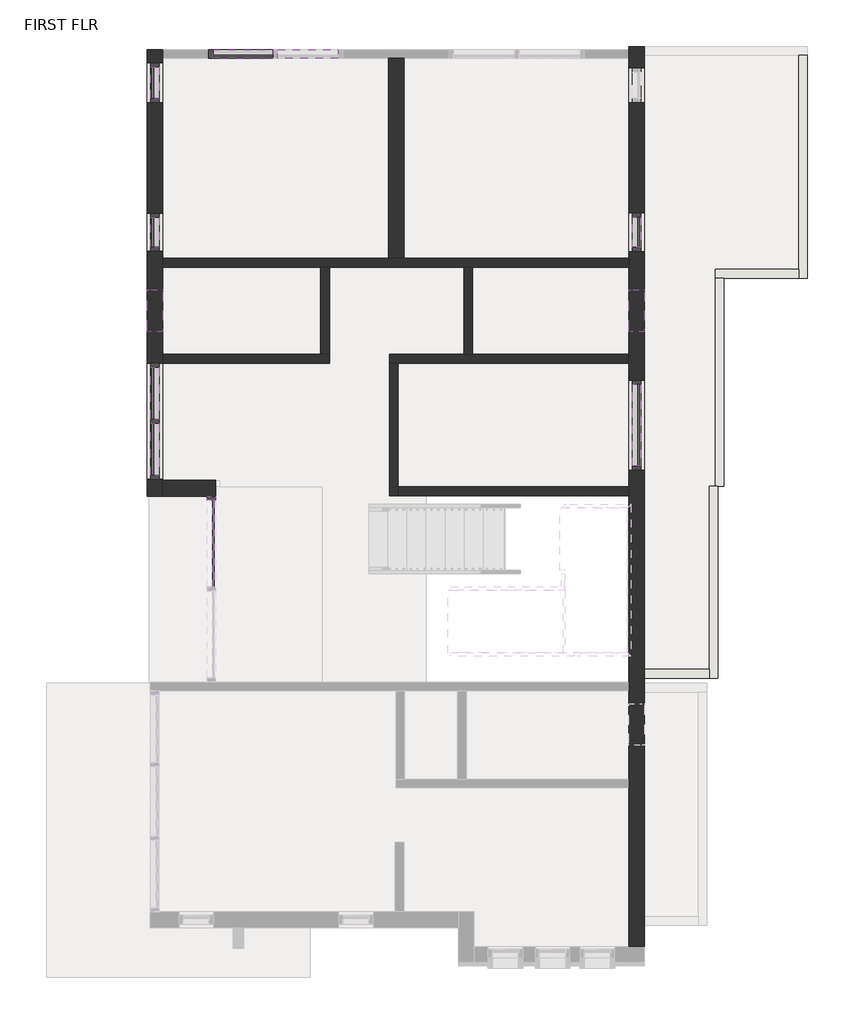
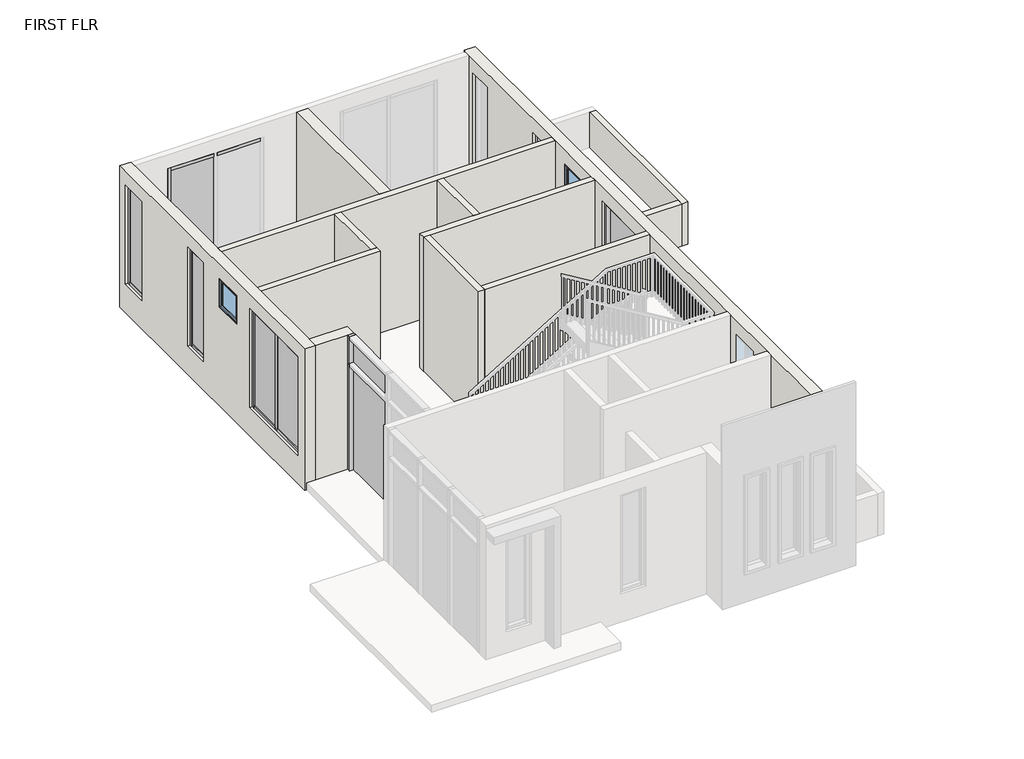
# One storey, part 2 of 4: 30 members, 16 walls, 9 plates, 2 windows.
"""IFC4 building model written with IfcOpenShell, lengths in millimetres."""

from ifc_helpers import new_model, si_unit, frame, origin, place, context, project, spatial, polyline, outline, extrude, faceted_brep, transform, mapped, element, save
from components import member_ee409385, member_2af3cda3, member_47bfaf8a, member_15823cb3, member_69a911c1, member_a3a7b6e3, member_bc7dbe04, member_83167d3d, member_3374d9b6, member_7cbddb58, member_5cd4c5ac, system_panel_glazed_2be43394, system_panel_glazed_82b35773, system_panel_glazed_a1cd5516, system_panel_glazed_0a3516e8, system_panel_glazed_a3b3c321, system_panel_glazed_660eca69, system_panel_glazed_3ab3cb8c, system_panel_glazed_6a2d4635, window_80340324

model = new_model("IFC4")

# Units and contexts
model_context = context("Model", 3, world=origin())
ifc_project = project(units=[si_unit("LENGTHUNIT", "METRE", prefix="MILLI")], contexts=[model_context])

# Site, building, storey
site = spatial("IfcSite", under=ifc_project)
building = spatial("IfcBuilding", under=site)
storey = spatial("IfcBuildingStorey", under=building, Name="FIRST FLR", Elevation=3048.0)

# Members
placement = place(None, origin())
member_shape = member_ee409385(model_context)
element("IfcMember", 1, ObjectType="Rectangular Mullion : 2.5\" x 5\" rectangular", at=placement, inside=storey, context=model_context, shape_type="MappedRepresentation", body=[
    mapped(member_shape, transform((-12015.640556, -5260.3016611, 5486.4), x_axis=(0.0, 1.0, 0.0), y_axis=(-1.0, 0.0, 0.0), z_axis=(0.0, 0.0, 1.0))),
])
member_2_shape = member_2af3cda3(model_context)
element("IfcMember", 2, ObjectType="Rectangular Mullion : 2.5\" x 5\" rectangular", at=placement, inside=storey, context=model_context, shape_type="MappedRepresentation", body=[
    mapped(member_2_shape, transform((-12015.640556, -5323.8016611, 3048.0), x_axis=(0.0, 0.0, -1.0), y_axis=(-1.0, 0.0, 0.0), z_axis=(0.0, 1.0, 0.0))),
])
member_3_shape = member_47bfaf8a(model_context)
element("IfcMember", 3, ObjectType="Rectangular Mullion : 2.5\" x 5\" rectangular", at=placement, inside=storey, context=model_context, shape_type="MappedRepresentation", body=[
    mapped(member_3_shape, transform((-12015.640556, -5260.3016611, 6096.0), x_axis=(0.0, 1.0, 0.0), y_axis=(-1.0, 0.0, 0.0), z_axis=(0.0, 0.0, 1.0))),
])
member_4_shape = member_15823cb3(model_context)
element("IfcMember", 4, ObjectType="Rectangular Mullion : 2.5\" x 5\" rectangular", at=placement, inside=storey, context=model_context, shape_type="MappedRepresentation", body=[
    mapped(member_4_shape, transform((-12841.140556, 556.2983389, 5791.2), x_axis=(0.0, 0.0, 1.0), y_axis=(-1.0, 0.0, 0.0), z_axis=(0.0, -1.0, 0.0))),
])
element("IfcMember", 5, ObjectType="Rectangular Mullion : 2.5\" x 5\" rectangular", at=placement, inside=storey, context=model_context, shape_type="MappedRepresentation", body=[
    mapped(member_4_shape, transform((-12841.140556, 1013.4983389, 3657.6), x_axis=(0.0, 0.0, -1.0), y_axis=(-1.0, 0.0, 0.0), z_axis=(0.0, 1.0, 0.0))),
])
member_5_shape = member_69a911c1(model_context)
element("IfcMember", 6, ObjectType="Rectangular Mullion : 2.5\" x 5\" rectangular", at=placement, inside=storey, context=model_context, shape_type="MappedRepresentation", body=[
    mapped(member_5_shape, transform((-12841.140556, -1617.3738817, 5791.2), x_axis=(0.0, 0.0, 1.0), y_axis=(-1.0, 0.0, 0.0), z_axis=(0.0, -1.0, 0.0))),
])
element("IfcMember", 7, ObjectType="Rectangular Mullion : 2.5\" x 5\" rectangular", at=placement, inside=storey, context=model_context, shape_type="MappedRepresentation", body=[
    mapped(member_5_shape, transform((-12841.140556, -1185.5738817, 3657.6), x_axis=(0.0, 0.0, -1.0), y_axis=(-1.0, 0.0, 0.0), z_axis=(0.0, 1.0, 0.0))),
])
member_6_shape = member_a3a7b6e3(model_context)
element("IfcMember", 8, ObjectType="Rectangular Mullion : 2.5\" x 5\" rectangular", at=placement, inside=storey, context=model_context, shape_type="MappedRepresentation", body=[
    mapped(member_6_shape, transform((-12841.140556, -4953.7451712, 5791.2), x_axis=(0.0, 0.0, 1.0), y_axis=(-1.0, 0.0, 0.0), z_axis=(0.0, -1.0, 0.0))),
])
element("IfcMember", 9, ObjectType="Rectangular Mullion : 2.5\" x 5\" rectangular", at=placement, inside=storey, context=model_context, shape_type="MappedRepresentation", body=[
    mapped(member_6_shape, transform((-12841.140556, -4134.5951712, 5791.2), x_axis=(0.0, 0.0, 1.0), y_axis=(-1.0, 0.0, 0.0), z_axis=(0.0, -1.0, 0.0))),
])
element("IfcMember", 10, ObjectType="Rectangular Mullion : 2.5\" x 5\" rectangular", at=placement, inside=storey, context=model_context, shape_type="MappedRepresentation", body=[
    mapped(member_6_shape, transform((-12841.140556, -3378.9451712, 3657.6), x_axis=(0.0, 0.0, -1.0), y_axis=(-1.0, 0.0, 0.0), z_axis=(0.0, 1.0, 0.0))),
])
element("IfcMember", 11, ObjectType="Rectangular Mullion : 2.5\" x 5\" rectangular", at=placement, inside=storey, context=model_context, shape_type="MappedRepresentation", body=[
    mapped(member_6_shape, transform((-12841.140556, -4198.0951712, 3657.6), x_axis=(0.0, 0.0, -1.0), y_axis=(-1.0, 0.0, 0.0), z_axis=(0.0, 1.0, 0.0))),
])
member_7_shape = member_bc7dbe04(model_context)
element("IfcMember", 12, ObjectType="Rectangular Mullion : 2.5\" x 5\" rectangular", at=placement, inside=storey, context=model_context, shape_type="MappedRepresentation", body=[
    mapped(member_7_shape, transform((-5795.8906521, -1625.1830995, 5791.2), x_axis=(0.0, 0.0, 1.0), y_axis=(-1.0, 0.0, 0.0), z_axis=(0.0, -1.0, 0.0))),
])
element("IfcMember", 13, ObjectType="Rectangular Mullion : 2.5\" x 5\" rectangular", at=placement, inside=storey, context=model_context, shape_type="MappedRepresentation", body=[
    mapped(member_7_shape, transform((-5795.8906521, -1180.6830995, 3657.6), x_axis=(0.0, 0.0, -1.0), y_axis=(-1.0, 0.0, 0.0), z_axis=(0.0, 1.0, 0.0))),
])
member_8_shape = member_83167d3d(model_context)
element("IfcMember", 14, ObjectType="Rectangular Mullion : 2.5\" x 5\" rectangular", at=placement, inside=storey, context=model_context, shape_type="MappedRepresentation", body=[
    mapped(member_8_shape, transform((-5795.8906521, -3626.5951712, 5791.2), x_axis=(0.0, 0.0, 1.0), y_axis=(1.0, 0.0, 0.0), z_axis=(0.0, 1.0, 0.0))),
])
element("IfcMember", 15, ObjectType="Rectangular Mullion : 2.5\" x 5\" rectangular", at=placement, inside=storey, context=model_context, shape_type="MappedRepresentation", body=[
    mapped(member_8_shape, transform((-5795.8906521, -4820.3951712, 3657.6), x_axis=(0.0, 0.0, -1.0), y_axis=(1.0, 0.0, 0.0), z_axis=(0.0, -1.0, 0.0))),
])
member_9_shape = member_3374d9b6(model_context)
element("IfcMember", 16, ObjectType="Rectangular Mullion : 2.5\" x 5\" rectangular", at=placement, inside=storey, context=model_context, shape_type="MappedRepresentation", body=[
    mapped(member_9_shape, transform((-12841.140556, 492.7983389, 3657.6), x_axis=(0.0, -1.0, 0.0), y_axis=(-1.0, 0.0, 0.0), z_axis=(0.0, 0.0, -1.0))),
])
element("IfcMember", 17, ObjectType="Rectangular Mullion : 2.5\" x 5\" rectangular", at=placement, inside=storey, context=model_context, shape_type="MappedRepresentation", body=[
    mapped(member_9_shape, transform((-12841.140556, -1680.8738817, 3657.6), x_axis=(0.0, -1.0, 0.0), y_axis=(-1.0, 0.0, 0.0), z_axis=(0.0, 0.0, -1.0))),
])
element("IfcMember", 18, ObjectType="Rectangular Mullion : 2.5\" x 5\" rectangular", at=placement, inside=storey, context=model_context, shape_type="MappedRepresentation", body=[
    mapped(member_9_shape, transform((-12841.140556, -5017.2451712, 3657.6), x_axis=(0.0, -1.0, 0.0), y_axis=(-1.0, 0.0, 0.0), z_axis=(0.0, 0.0, -1.0))),
])
element("IfcMember", 19, ObjectType="Rectangular Mullion : 2.5\" x 5\" rectangular", at=placement, inside=storey, context=model_context, shape_type="MappedRepresentation", body=[
    mapped(member_9_shape, transform((-5795.8906521, -3563.0951712, 3657.6), x_axis=(0.0, 1.0, 0.0), y_axis=(1.0, 0.0, 0.0), z_axis=(0.0, 0.0, -1.0))),
])
element("IfcMember", 20, ObjectType="Rectangular Mullion : 2.5\" x 5\" rectangular", at=placement, inside=storey, context=model_context, shape_type="MappedRepresentation", body=[
    mapped(member_9_shape, transform((-12841.140556, 1076.9983389, 5791.2), x_axis=(0.0, 1.0, 0.0), y_axis=(-1.0, 0.0, 0.0), z_axis=(0.0, 0.0, 1.0))),
])
element("IfcMember", 21, ObjectType="Rectangular Mullion : 2.5\" x 5\" rectangular", at=placement, inside=storey, context=model_context, shape_type="MappedRepresentation", body=[
    mapped(member_9_shape, transform((-12841.140556, -1122.0738817, 5791.2), x_axis=(0.0, 1.0, 0.0), y_axis=(-1.0, 0.0, 0.0), z_axis=(0.0, 0.0, 1.0))),
])
element("IfcMember", 22, ObjectType="Rectangular Mullion : 2.5\" x 5\" rectangular", at=placement, inside=storey, context=model_context, shape_type="MappedRepresentation", body=[
    mapped(member_9_shape, transform((-12841.140556, -3315.4451712, 5791.2), x_axis=(0.0, 1.0, 0.0), y_axis=(-1.0, 0.0, 0.0), z_axis=(0.0, 0.0, 1.0))),
])
element("IfcMember", 23, ObjectType="Rectangular Mullion : 2.5\" x 5\" rectangular", at=placement, inside=storey, context=model_context, shape_type="MappedRepresentation", body=[
    mapped(member_9_shape, transform((-5795.8906521, -4883.8951712, 5791.2), x_axis=(0.0, -1.0, 0.0), y_axis=(1.0, 0.0, 0.0), z_axis=(0.0, 0.0, 1.0))),
])
member_10_shape = member_7cbddb58(model_context)
element("IfcMember", 24, ObjectType="Rectangular Mullion : 2.5\" x 5\" rectangular", at=placement, inside=storey, context=model_context, shape_type="MappedRepresentation", body=[
    mapped(member_10_shape, transform((-12841.140556, -4166.3451712, 3657.6), x_axis=(0.0, -1.0, 0.0), y_axis=(-1.0, 0.0, 0.0), z_axis=(0.0, 0.0, -1.0))),
])
element("IfcMember", 25, ObjectType="Rectangular Mullion : 2.5\" x 5\" rectangular", at=placement, inside=storey, context=model_context, shape_type="MappedRepresentation", body=[
    mapped(member_9_shape, transform((-5795.8906521, -1688.6830995, 3657.6), x_axis=(0.0, -1.0, 0.0), y_axis=(-1.0, 0.0, 0.0), z_axis=(0.0, 0.0, -1.0))),
])
element("IfcMember", 26, ObjectType="Rectangular Mullion : 2.5\" x 5\" rectangular", at=placement, inside=storey, context=model_context, shape_type="MappedRepresentation", body=[
    mapped(member_9_shape, transform((-12054.1911408, 1203.9983389, 3657.6), x_axis=(-1.0, 0.0, 0.0), y_axis=(0.0, 1.0, 0.0), z_axis=(0.0, 0.0, -1.0))),
])
element("IfcMember", 27, ObjectType="Rectangular Mullion : 2.5\" x 5\" rectangular", at=placement, inside=storey, context=model_context, shape_type="MappedRepresentation", body=[
    mapped(member_9_shape, transform((-5795.8906521, -1117.1830995, 5791.2), x_axis=(0.0, 1.0, 0.0), y_axis=(-1.0, 0.0, 0.0), z_axis=(0.0, 0.0, 1.0))),
])
member_11_shape = member_5cd4c5ac(model_context)
element("IfcMember", 28, ObjectType="Rectangular Mullion : 2.5\" x 5\" rectangular", at=placement, inside=storey, context=model_context, shape_type="MappedRepresentation", body=[
    mapped(member_11_shape, transform((-11990.6911408, 1203.9983389, 5791.2), x_axis=(0.0, 0.0, 1.0), y_axis=(0.0, 1.0, 0.0), z_axis=(-1.0, 0.0, 0.0))),
])
element("IfcMember", 29, ObjectType="Rectangular Mullion : 2.5\" x 5\" rectangular", at=placement, inside=storey, context=model_context, shape_type="MappedRepresentation", body=[
    mapped(member_11_shape, transform((-11044.5411408, 1203.9983389, 5791.2), x_axis=(0.0, 0.0, 1.0), y_axis=(0.0, 1.0, 0.0), z_axis=(-1.0, 0.0, 0.0))),
])
element("IfcMember", 30, ObjectType="Rectangular Mullion : 2.5\" x 5\" rectangular", at=placement, inside=storey, context=model_context, shape_type="MappedRepresentation", body=[
    mapped(member_11_shape, transform((-11108.0411408, 1203.9983389, 3657.6), x_axis=(0.0, 0.0, -1.0), y_axis=(0.0, 1.0, 0.0), z_axis=(1.0, 0.0, 0.0))),
])

# Plates
system_panel_glazed_shape = system_panel_glazed_2be43394(model_context)
element("IfcPlate", 31, ObjectType="System Panel : Glazed", at=placement, inside=storey, context=model_context, shape_type="MappedRepresentation", body=[
    mapped(system_panel_glazed_shape, transform((-12015.640556, -5955.8340156, 3111.5), x_axis=(0.0, -1.0, 0.0), y_axis=(1.0, 0.0, 0.0), z_axis=(0.0, 0.0, 1.0))),
])
system_panel_glazed_2_shape = system_panel_glazed_82b35773(model_context)
element("IfcPlate", 32, ObjectType="System Panel : Glazed", at=placement, inside=storey, context=model_context, shape_type="MappedRepresentation", body=[
    mapped(system_panel_glazed_2_shape, transform((-12015.640556, -5955.8340156, 5518.15), x_axis=(0.0, -1.0, 0.0), y_axis=(1.0, 0.0, 0.0), z_axis=(0.0, 0.0, 1.0))),
])
system_panel_glazed_3_shape = system_panel_glazed_a1cd5516(model_context)
element("IfcPlate", 33, ObjectType="System Panel : Glazed", at=placement, inside=storey, context=model_context, shape_type="MappedRepresentation", body=[
    mapped(system_panel_glazed_3_shape, transform((-12841.140556, 784.8983389, 3721.1), x_axis=(0.0, -1.0, 0.0), y_axis=(1.0, 0.0, 0.0), z_axis=(0.0, 0.0, 1.0))),
])
system_panel_glazed_4_shape = system_panel_glazed_0a3516e8(model_context)
element("IfcPlate", 34, ObjectType="System Panel : Glazed", at=placement, inside=storey, context=model_context, shape_type="MappedRepresentation", body=[
    mapped(system_panel_glazed_4_shape, transform((-12841.140556, -1401.4738817, 3721.1), x_axis=(0.0, -1.0, 0.0), y_axis=(1.0, 0.0, 0.0), z_axis=(0.0, 0.0, 1.0))),
])
system_panel_glazed_5_shape = system_panel_glazed_a3b3c321(model_context)
element("IfcPlate", 35, ObjectType="System Panel : Glazed", at=placement, inside=storey, context=model_context, shape_type="MappedRepresentation", body=[
    mapped(system_panel_glazed_5_shape, transform((-12841.140556, -3756.7701712, 3721.1), x_axis=(0.0, -1.0, 0.0), y_axis=(1.0, 0.0, 0.0), z_axis=(0.0, 0.0, 1.0))),
])
element("IfcPlate", 36, ObjectType="System Panel : Glazed", at=placement, inside=storey, context=model_context, shape_type="MappedRepresentation", body=[
    mapped(system_panel_glazed_5_shape, transform((-12841.140556, -4575.9201712, 3721.1), x_axis=(0.0, -1.0, 0.0), y_axis=(1.0, 0.0, 0.0), z_axis=(0.0, 0.0, 1.0))),
])
system_panel_glazed_6_shape = system_panel_glazed_660eca69(model_context)
element("IfcPlate", 37, ObjectType="System Panel : Glazed", at=placement, inside=storey, context=model_context, shape_type="MappedRepresentation", body=[
    mapped(system_panel_glazed_6_shape, transform((-5795.8906521, -1402.9330995, 3721.1), x_axis=(0.0, -1.0, 0.0), y_axis=(1.0, 0.0, 0.0), z_axis=(0.0, 0.0, 1.0))),
])
system_panel_glazed_7_shape = system_panel_glazed_3ab3cb8c(model_context)
element("IfcPlate", 38, ObjectType="System Panel : Glazed", at=placement, inside=storey, context=model_context, shape_type="MappedRepresentation", body=[
    mapped(system_panel_glazed_7_shape, transform((-11549.3661408, 1203.9983389, 3721.1), x_axis=(-1.0, 0.0, 0.0), y_axis=(0.0, -1.0, 0.0), z_axis=(0.0, 0.0, 1.0))),
])
system_panel_glazed_8_shape = system_panel_glazed_6a2d4635(model_context)
element("IfcPlate", 39, ObjectType="System Panel : Glazed", at=placement, inside=storey, context=model_context, shape_type="MappedRepresentation", body=[
    mapped(system_panel_glazed_8_shape, transform((-5795.8906521, -4223.4951712, 3721.1), x_axis=(0.0, 1.0, 0.0), y_axis=(-1.0, 0.0, 0.0), z_axis=(0.0, 0.0, 1.0))),
])

# Walls
element("IfcWall", 40, ObjectType="EXTERIOR WALL 9\"", at=placement, inside=storey, context=model_context, shape_type="Brep", body=[
    faceted_brep([(-12955.440556, 1267.4983389, 3048.0), (-12955.440556, -5260.3016611, 3048.0), (-12955.440556, -5260.3016611, 6096.0), (-12955.440556, 1267.4983389, 6096.0), (-12955.440556, 1076.9983389, 3657.6), (-12955.440556, 1076.9983389, 5791.2), (-12955.440556, 492.7983389, 5791.2), (-12955.440556, 492.7983389, 3657.6), (-12955.440556, -1122.0738817, 3657.6), (-12955.440556, -1122.0738817, 5791.2), (-12955.440556, -1680.8738817, 5791.2), (-12955.440556, -1680.8738817, 3657.6), (-12955.440556, -3315.4451712, 3657.6), (-12955.440556, -3315.4451712, 5791.2), (-12955.440556, -5017.2451712, 5791.2), (-12955.440556, -5017.2451712, 3657.6), (-12955.440556, -2245.4701712, 5791.2), (-12955.440556, -2855.0701712, 5791.2), (-12955.440556, -2855.0701712, 5181.6), (-12955.440556, -2245.4701712, 5181.6), (-12726.840556, -5260.3016611, 3048.0), (-12726.840556, -5031.7016611, 3048.0), (-12726.840556, -3315.4451712, 3048.0), (-12726.840556, -3188.4451712, 3048.0), (-12726.840556, -1912.0951712, 3048.0), (-12726.840556, -1785.0951712, 3048.0), (-12726.840556, 1140.4983389, 3048.0), (-12726.840556, 1267.4983389, 3048.0), (-12726.840556, 1267.4983389, 6096.0), (-12726.840556, 1140.4983389, 6096.0), (-12726.840556, -1785.0951712, 6096.0), (-12726.840556, -1912.0951712, 6096.0), (-12726.840556, -3188.4451712, 6096.0), (-12726.840556, -3315.4451712, 6096.0), (-12726.840556, -5031.7016611, 6096.0), (-12726.840556, -5260.3016611, 6096.0), (-12726.840556, 1076.9983389, 5791.2), (-12726.840556, 1076.9983389, 3657.6), (-12726.840556, 492.7983389, 3657.6), (-12726.840556, 492.7983389, 5791.2), (-12726.840556, -1122.0738817, 5791.2), (-12726.840556, -1122.0738817, 3657.6), (-12726.840556, -1680.8738817, 3657.6), (-12726.840556, -1680.8738817, 5791.2), (-12726.840556, -3315.4451712, 5791.2), (-12726.840556, -3315.4451712, 3657.6), (-12726.840556, -5017.2451712, 3657.6), (-12726.840556, -5017.2451712, 5791.2), (-12726.840556, -2245.4701712, 5791.2), (-12726.840556, -2245.4701712, 5181.6), (-12726.840556, -2855.0701712, 5181.6), (-12726.840556, -2855.0701712, 5791.2)], [[[0, 1, 2, 3], [4, 5, 6, 7], [8, 9, 10, 11], [12, 13, 14, 15], [16, 17, 18, 19]], [[20, 21, 22, 23, 24, 25, 26, 27, 28, 29, 30, 31, 32, 33, 34, 35], [36, 37, 38, 39], [40, 41, 42, 43], [44, 45, 46, 47], [48, 49, 50, 51]], [[1, 0, 27, 26, 25, 24, 23, 22, 21, 20]], [[3, 2, 35, 34, 33, 32, 31, 30, 29, 28]], [[2, 1, 20, 35]], [[0, 3, 28, 27]], [[36, 5, 4, 37]], [[5, 36, 39, 6]], [[6, 39, 38, 7]], [[37, 4, 7, 38]], [[8, 41, 40, 9]], [[9, 40, 43, 10]], [[10, 43, 42, 11]], [[41, 8, 11, 42]], [[12, 45, 44, 13]], [[13, 44, 47, 14]], [[46, 15, 14, 47]], [[45, 12, 15, 46]], [[49, 48, 16, 19]], [[50, 49, 19, 18]], [[51, 50, 18, 17]], [[48, 51, 17, 16]]]),
])
element("IfcWall", 41, ObjectType="EXTERIOR WALL 9\"", at=placement, inside=storey, context=model_context, shape_type="SweptSolid", body=[
    extrude(outline(polyline([(-11952.140556, -5260.3016611), (-12726.840556, -5260.3016611), (-12726.840556, -5031.7016611), (-11952.140556, -5031.7016611), (-11952.140556, -5260.3016611)])), frame((0.0, 0.0, 3048.0), z_axis=(0.0, 0.0, 1.0), x_axis=(1.0, 0.0, 0.0)), (0.0, 0.0, 1.0), 3048.0),
])
element("IfcWall", 42, ObjectType="EXTERIOR WALL 9\"", at=placement, inside=storey, context=model_context, shape_type="Brep", body=[
    faceted_brep([(-5681.5906521, -11847.6453012, 3048.0), (-5681.5906521, -11534.9310793, 3048.0), (-5681.5906521, -11407.9310793, 3048.0), (-5681.5906521, -8124.9810793, 3048.0), (-5681.5906521, -7997.9810793, 3048.0), (-5681.5906521, -7921.7810793, 3048.0), (-5681.5906521, -7794.7810793, 3048.0), (-5681.5906521, 1184.7951326, 3048.0), (-5681.5906521, 1311.7951326, 3048.0), (-5681.5906521, 1311.7951326, 3962.4), (-5681.5906521, 1311.7951326, 6096.0), (-5681.5906521, -11847.6453012, 6096.0), (-5681.5906521, 1000.7983389, 5791.2), (-5681.5906521, 1000.7983389, 3657.6), (-5681.5906521, 492.7983389, 3657.6), (-5681.5906521, 492.7983389, 5791.2), (-5681.5906521, -1117.1830995, 5791.2), (-5681.5906521, -1117.1830995, 3657.6), (-5681.5906521, -1688.6830995, 3657.6), (-5681.5906521, -1688.6830995, 5791.2), (-5681.5906521, -2245.4701712, 5791.2), (-5681.5906521, -2245.4701712, 5181.6), (-5681.5906521, -2855.0701712, 5181.6), (-5681.5906521, -2855.0701712, 5791.2), (-5681.5906521, -4883.8951712, 3657.6), (-5681.5906521, -4883.8951712, 5791.2), (-5681.5906521, -3563.0951712, 5791.2), (-5681.5906521, -3563.0951712, 3657.6), (-5681.5906521, -8906.0310793, 5791.2), (-5681.5906521, -8296.4310793, 5791.2), (-5681.5906521, -8296.4310793, 5181.6), (-5681.5906521, -8906.0310793, 5181.6), (-5910.1906521, 1311.7951326, 3048.0), (-5910.1906521, 1267.4983389, 3048.0), (-5910.1906521, 1140.4983389, 3048.0), (-5910.1906521, -1785.0951712, 3048.0), (-5910.1906521, -1912.0951712, 3048.0), (-5910.1906521, -3188.4451712, 3048.0), (-5910.1906521, -3315.4451712, 3048.0), (-5910.1906521, -5125.1951712, 3048.0), (-5910.1906521, -5252.1951712, 3048.0), (-5910.1906521, -7978.9310793, 3048.0), (-5910.1906521, -8105.9310793, 3048.0), (-5910.1906521, -9397.5830995, 3048.0), (-5910.1906521, -9524.5830995, 3048.0), (-5910.1906521, -11847.6453012, 3048.0), (-5910.1906521, -11847.6453012, 6096.0), (-5910.1906521, -9524.5830995, 6096.0), (-5910.1906521, -9397.5830995, 6096.0), (-5910.1906521, -8105.9310793, 6096.0), (-5910.1906521, -7978.9310793, 6096.0), (-5910.1906521, -5252.1951712, 6096.0), (-5910.1906521, -5125.1951712, 6096.0), (-5910.1906521, -3315.4451712, 6096.0), (-5910.1906521, -3188.4451712, 6096.0), (-5910.1906521, -1912.0951712, 6096.0), (-5910.1906521, -1785.0951712, 6096.0), (-5910.1906521, 1140.4983389, 6096.0), (-5910.1906521, 1267.4983389, 6096.0), (-5910.1906521, 1311.7951326, 6096.0), (-5910.1906521, 1000.7983389, 3657.6), (-5910.1906521, 1000.7983389, 5791.2), (-5910.1906521, 492.7983389, 5791.2), (-5910.1906521, 492.7983389, 3657.6), (-5910.1906521, -1117.1830995, 3657.6), (-5910.1906521, -1117.1830995, 5791.2), (-5910.1906521, -1688.6830995, 5791.2), (-5910.1906521, -1688.6830995, 3657.6), (-5910.1906521, -2245.4701712, 5791.2), (-5910.1906521, -2855.0701712, 5791.2), (-5910.1906521, -2855.0701712, 5181.6), (-5910.1906521, -2245.4701712, 5181.6), (-5910.1906521, -4883.8951712, 5791.2), (-5910.1906521, -4883.8951712, 3657.6), (-5910.1906521, -3563.0951712, 3657.6), (-5910.1906521, -3563.0951712, 5791.2), (-5910.1906521, -8906.0310793, 5791.2), (-5910.1906521, -8906.0310793, 5181.6), (-5910.1906521, -8296.4310793, 5181.6), (-5910.1906521, -8296.4310793, 5791.2)], [[[0, 1, 2, 3, 4, 5, 6, 7, 8, 9, 10, 11], [12, 13, 14, 15], [16, 17, 18, 19], [20, 21, 22, 23], [24, 25, 26, 27], [28, 29, 30, 31]], [[32, 33, 34, 35, 36, 37, 38, 39, 40, 41, 42, 43, 44, 45, 46, 47, 48, 49, 50, 51, 52, 53, 54, 55, 56, 57, 58, 59], [60, 61, 62, 63], [64, 65, 66, 67], [68, 69, 70, 71], [72, 73, 74, 75], [76, 77, 78, 79]], [[8, 7, 6, 5, 4, 3, 2, 1, 0, 45, 44, 43, 42, 41, 40, 39, 38, 37, 36, 35, 34, 33, 32]], [[11, 10, 59, 58, 57, 56, 55, 54, 53, 52, 51, 50, 49, 48, 47, 46]], [[0, 11, 46, 45]], [[12, 61, 60, 13]], [[61, 12, 15, 62]], [[62, 15, 14, 63]], [[13, 60, 63, 14]], [[64, 17, 16, 65]], [[65, 16, 19, 66]], [[66, 19, 18, 67]], [[17, 64, 67, 18]], [[21, 20, 68, 71]], [[22, 21, 71, 70]], [[23, 22, 70, 69]], [[20, 23, 69, 68]], [[72, 25, 24, 73]], [[25, 72, 75, 26]], [[26, 75, 74, 27]], [[73, 24, 27, 74]], [[77, 76, 28, 31]], [[78, 77, 31, 30]], [[79, 78, 30, 29]], [[76, 79, 29, 28]], [[10, 9, 8, 32, 59]]]),
])
element("IfcWall", 43, ObjectType="EXTERIOR WALL 9\"", at=placement, inside=storey, context=model_context, shape_type="SweptSolid", body=[
    extrude(outline(polyline([(-9425.2911408, -1785.0951712), (-9425.2911408, 1140.4983389), (-9196.6911408, 1140.4983389), (-9196.6911408, -1785.0951712), (-9425.2911408, -1785.0951712)])), frame((0.0, 0.0, 3048.0), z_axis=(0.0, 0.0, 1.0), x_axis=(1.0, 0.0, 0.0)), (0.0, 0.0, 1.0), 3048.0),
])
element("IfcWall", 44, ObjectType="INTERIOR WALL PAINT 5\"", at=placement, inside=storey, context=model_context, shape_type="Brep", body=[
    faceted_brep([(-12726.840556, -1912.0951712, 3048.0), (-10415.440556, -1912.0951712, 3048.0), (-10288.440556, -1912.0951712, 3048.0), (-8320.3911408, -1912.0951712, 3048.0), (-8193.3911408, -1912.0951712, 3048.0), (-5910.1906521, -1912.0951712, 3048.0), (-5910.1906521, -1912.0951712, 6096.0), (-8193.3911408, -1912.0951712, 6096.0), (-8320.3911408, -1912.0951712, 6096.0), (-10288.440556, -1912.0951712, 6096.0), (-10415.440556, -1912.0951712, 6096.0), (-12726.840556, -1912.0951712, 6096.0), (-12726.840556, -1785.0951712, 3048.0), (-12726.840556, -1785.0951712, 6096.0), (-9425.2911408, -1785.0951712, 6096.0), (-9196.6911408, -1785.0951712, 6096.0), (-5910.1906521, -1785.0951712, 6096.0), (-5910.1906521, -1785.0951712, 3048.0), (-9196.6911408, -1785.0951712, 3048.0), (-9425.2911408, -1785.0951712, 3048.0)], [[[0, 1, 2, 3, 4, 5, 6, 7, 8, 9, 10, 11]], [[12, 13, 14, 15, 16, 17, 18, 19]], [[5, 4, 3, 2, 1, 0, 12, 19, 18, 17]], [[11, 10, 9, 8, 7, 6, 16, 15, 14, 13]], [[0, 11, 13, 12]], [[6, 5, 17, 16]]]),
])
element("IfcWall", 45, ObjectType="INTERIOR WALL PAINT 5\"", at=placement, inside=storey, context=model_context, shape_type="Brep", body=[
    faceted_brep([(-12726.840556, -3315.4451712, 3048.0), (-10288.440556, -3315.4451712, 3048.0), (-10288.440556, -3315.4451712, 6096.0), (-12726.840556, -3315.4451712, 6096.0), (-12726.840556, -3188.4451712, 3048.0), (-12726.840556, -3188.4451712, 6096.0), (-10415.440556, -3188.4451712, 6096.0), (-10288.440556, -3188.4451712, 6096.0), (-10288.440556, -3188.4451712, 3048.0), (-10415.440556, -3188.4451712, 3048.0)], [[[0, 1, 2, 3]], [[4, 5, 6, 7, 8, 9]], [[1, 0, 4, 9, 8]], [[3, 2, 7, 6, 5]], [[0, 3, 5, 4]], [[2, 1, 8, 7]]]),
])
element("IfcWall", 46, ObjectType="INTERIOR WALL PAINT 5\"", at=placement, inside=storey, context=model_context, shape_type="SweptSolid", body=[
    extrude(outline(polyline([(-10288.440556, -1912.0951712), (-10288.440556, -3188.4451712), (-10415.440556, -3188.4451712), (-10415.440556, -1912.0951712), (-10288.440556, -1912.0951712)])), frame((0.0, 0.0, 3048.0), z_axis=(0.0, 0.0, 1.0), x_axis=(1.0, 0.0, 0.0)), (0.0, 0.0, 1.0), 3048.0),
])
element("IfcWall", 47, ObjectType="INTERIOR WALL PAINT 5\"", at=placement, inside=storey, context=model_context, shape_type="Brep", body=[
    faceted_brep([(-5910.1906521, -3188.4451712, 3048.0), (-8193.3911408, -3188.4451712, 3048.0), (-8320.3911408, -3188.4451712, 3048.0), (-9409.0406521, -3188.4451712, 3048.0), (-9409.0406521, -3188.4451712, 6096.0), (-8320.3911408, -3188.4451712, 6096.0), (-8193.3911408, -3188.4451712, 6096.0), (-5910.1906521, -3188.4451712, 6096.0), (-5910.1906521, -3315.4451712, 3048.0), (-5910.1906521, -3315.4451712, 6096.0), (-9282.0406521, -3315.4451712, 6096.0), (-9409.0406521, -3315.4451712, 6096.0), (-9409.0406521, -3315.4451712, 3048.0), (-9282.0406521, -3315.4451712, 3048.0)], [[[0, 1, 2, 3, 4, 5, 6, 7]], [[8, 9, 10, 11, 12, 13]], [[3, 2, 1, 0, 8, 13, 12]], [[7, 6, 5, 4, 11, 10, 9]], [[0, 7, 9, 8]], [[4, 3, 12, 11]]]),
])
element("IfcWall", 48, ObjectType="INTERIOR WALL PAINT 5\"", at=placement, inside=storey, context=model_context, shape_type="SweptSolid", body=[
    extrude(outline(polyline([(-8320.3911408, -3188.4451712), (-8320.3911408, -1912.0951712), (-8193.3911408, -1912.0951712), (-8193.3911408, -3188.4451712), (-8320.3911408, -3188.4451712)])), frame((0.0, 0.0, 3048.0), z_axis=(0.0, 0.0, 1.0), x_axis=(1.0, 0.0, 0.0)), (0.0, 0.0, 1.0), 3048.0),
])
element("IfcWall", 49, ObjectType="INTERIOR WALL PAINT 5\"", at=placement, inside=storey, context=model_context, shape_type="Brep", body=[
    faceted_brep([(-9409.0406521, -3315.4451712, 3048.0), (-9409.0406521, -5252.1951712, 3048.0), (-9409.0406521, -5252.1951712, 6096.0), (-9409.0406521, -3315.4451712, 6096.0), (-9282.0406521, -3315.4451712, 3048.0), (-9282.0406521, -3315.4451712, 6096.0), (-9282.0406521, -5125.1951712, 6096.0), (-9282.0406521, -5252.1951712, 6096.0), (-9282.0406521, -5252.1951712, 3048.0), (-9282.0406521, -5125.1951712, 3048.0)], [[[0, 1, 2, 3]], [[4, 5, 6, 7, 8, 9]], [[1, 0, 4, 9, 8]], [[3, 2, 7, 6, 5]], [[0, 3, 5, 4]], [[2, 1, 8, 7]]]),
])
element("IfcWall", 50, ObjectType="INTERIOR WALL PAINT 5\"", at=placement, inside=storey, context=model_context, shape_type="SweptSolid", body=[
    extrude(outline(polyline([(-5910.1906521, -5252.1951712), (-9282.0406521, -5252.1951712), (-9282.0406521, -5125.1951712), (-5910.1906521, -5125.1951712), (-5910.1906521, -5252.1951712)])), frame((0.0, 0.0, 3048.0), z_axis=(0.0, 0.0, 1.0), x_axis=(1.0, 0.0, 0.0)), (0.0, 0.0, 1.0), 3048.0),
])
element("IfcWall", 51, ObjectType="INTERIOR WALL PAINT 5\"", at=placement, inside=storey, context=model_context, shape_type="Brep", body=[
    faceted_brep([(-3424.4727979, 1184.7951326, 3048.0), (-3424.4727979, -1944.8337491, 3048.0), (-3424.4727979, -2071.8337491, 3048.0), (-3424.4727979, -2071.8337491, 3962.4), (-3424.4727979, -1944.8337491, 3962.4), (-3424.4727979, 1184.7951326, 3962.4), (-3297.4727979, 1184.7951326, 3048.0), (-3297.4727979, 1184.7951326, 3962.4), (-3297.4727979, -2071.8337491, 3962.4), (-3297.4727979, -2071.8337491, 3048.0)], [[[0, 1, 2, 3, 4, 5]], [[6, 7, 8, 9]], [[2, 1, 0, 6, 9]], [[5, 4, 3, 8, 7]], [[0, 5, 7, 6]], [[3, 2, 9, 8]]]),
])
element("IfcWall", 52, ObjectType="INTERIOR WALL PAINT 5\"", at=placement, inside=storey, context=model_context, shape_type="Brep", body=[
    faceted_brep([(-3424.4727979, -1944.8337491, 3048.0), (-4643.6727979, -1944.8337491, 3048.0), (-4643.6727979, -1944.8337491, 3962.4), (-3424.4727979, -1944.8337491, 3962.4), (-3424.4727979, -2071.8337491, 3048.0), (-3424.4727979, -2071.8337491, 3962.4), (-4516.6727979, -2071.8337491, 3962.4), (-4643.6727979, -2071.8337491, 3962.4), (-4643.6727979, -2071.8337491, 3048.0), (-4516.6727979, -2071.8337491, 3048.0)], [[[0, 1, 2, 3]], [[4, 5, 6, 7, 8, 9]], [[1, 0, 4, 9, 8]], [[3, 2, 7, 6, 5]], [[0, 3, 5, 4]], [[2, 1, 8, 7]]]),
])
element("IfcWall", 53, ObjectType="INTERIOR WALL PAINT 5\"", at=placement, inside=storey, context=model_context, shape_type="Brep", body=[
    faceted_brep([(-4643.6727979, -2071.8337491, 3048.0), (-4643.6727979, -5119.6951024, 3048.0), (-4643.6727979, -5119.6951024, 3962.4), (-4643.6727979, -2071.8337491, 3962.4), (-4516.6727979, -2071.8337491, 3048.0), (-4516.6727979, -2071.8337491, 3962.4), (-4516.6727979, -5119.6951024, 3962.4), (-4516.6727979, -5119.6951024, 3048.0), (-4605.5727979, -5119.6951024, 3048.0), (-4605.5727979, -5119.6951024, 3962.4)], [[[0, 1, 2, 3]], [[4, 5, 6, 7]], [[1, 0, 4, 7, 8]], [[2, 1, 8, 7, 6, 9]], [[3, 2, 9, 6, 5]], [[0, 3, 5, 4]]]),
])
element("IfcWall", 54, ObjectType="INTERIOR WALL PAINT 5\"", at=placement, inside=storey, context=model_context, shape_type="Brep", body=[
    faceted_brep([(-4732.5727979, -5119.6951024, 3048.0), (-4732.5727979, -7794.7810793, 3048.0), (-4732.5727979, -7921.7810793, 3048.0), (-4732.5727979, -7921.7810793, 3962.4), (-4732.5727979, -7794.7810793, 3962.4), (-4732.5727979, -5119.6951024, 3962.4), (-4605.5727979, -5119.6951024, 3048.0), (-4605.5727979, -5119.6951024, 3962.4), (-4605.5727979, -7921.7810793, 3962.4), (-4605.5727979, -7921.7810793, 3048.0), (-4643.6727979, -5119.6951024, 3048.0), (-4643.6727979, -5119.6951024, 3962.4)], [[[0, 1, 2, 3, 4, 5]], [[6, 7, 8, 9]], [[2, 1, 0, 10, 6, 9]], [[5, 4, 3, 8, 7, 11]], [[0, 5, 11, 7, 6, 10]], [[3, 2, 9, 8]]]),
])
element("IfcWall", 55, ObjectType="INTERIOR WALL PAINT 5\"", at=placement, inside=storey, context=model_context, shape_type="SweptSolid", body=[
    extrude(outline(polyline([(-5681.5906521, -7794.7810793), (-4732.5727979, -7794.7810793), (-4732.5727979, -7921.7810793), (-5681.5906521, -7921.7810793), (-5681.5906521, -7794.7810793)])), frame((0.0, 0.0, 3048.0), z_axis=(0.0, 0.0, 1.0), x_axis=(1.0, 0.0, 0.0)), (0.0, 0.0, 1.0), 914.4),
])

# Windows
window_shape = window_80340324(model_context)
element("IfcWindow", 56, ObjectType="Fixed : 24\" x 24\"", at=placement, inside=storey, context=model_context, shape_type="MappedRepresentation", body=[
    mapped(window_shape, transform((-5795.8906521, -2512.1701712, 4267.2), x_axis=(0.0, 1.0, 0.0), y_axis=(-1.0, 0.0, 0.0), z_axis=(0.0, 0.0, 1.0))),
])
element("IfcWindow", 57, ObjectType="Fixed : 24\" x 24\"", at=placement, inside=storey, context=model_context, shape_type="MappedRepresentation", body=[
    mapped(window_shape, transform((-12841.140556, -2512.1701712, 4267.2), x_axis=(0.0, 1.0, 0.0), y_axis=(-1.0, 0.0, 0.0), z_axis=(0.0, 0.0, 1.0))),
])

save(model, "model.ifc")

# Revit data of these elements
# Type "Rectangular Mullion : 2.5\" x 5\" rectangular"
#   built-in parameter 1007304 = 0.416667 (stored number, unit not read)
#   built-in parameter 1007301 = 0.104167 (stored number, unit not read)
#   built-in parameter 1007300 = 0.104167 (stored number, unit not read)
# Type "System Panel : Glazed"
#   Construction Type Id = "GSP4R"
#   Analytic Construction = "1/8 in Pilkington single glazing"
#   Visual Light Transmittance = 0.9
#   Solar Heat Gain Coefficient = 0.86
#   Heat Transfer Coefficient (U) = 1.18115 BTU/(h·ft²·°F)
#   Define Thermal Properties by = 1
# Type "EXTERIOR WALL 9\""
#   Assembly Code = "B2010"
#   Layers, outside or top first: 0' - 9" "EXTERIOR WALL PAINT" (function 1)
# Type "INTERIOR WALL PAINT 5\""
#   Assembly Code = "B2010"
#   Layers, outside or top first: 0' - 5" "EXTERIOR WALL PAINT" (function 1)
# Type "Fixed : 24\" x 24\""
#   Type Mark = "3"
#   Construction Type Id = "GSP4R"
#   Assembly Code = "B2020100"
#   Analytic Construction = "1/8 in Pilkington single glazing"
#   Visual Light Transmittance = 0.9
#   Solar Heat Gain Coefficient = 0.78
#   Heat Transfer Coefficient (U) = 0.6496 BTU/(h·ft²·°F)
#   Height = 2' - 0"
#   Default Sill Height = 3' - 0"
#   Width = 2' - 0"
#   Window Inset = 0' - 0 3/4"
#   Define Thermal Properties by = 1
#   Define Thermal Properties by = 1
#   Glass Pane Material = Glass
#   Sash Material = Sash
#   Wall Closure = (empty or 0)
# Elements 1, 2, 3, 4, 5, 6, 7, 8, 9, 10, 11, 12, 13, 14, 15, 16, 17, 18, 19, 20, 21, 22, 23, 24, 25, 26, 27, 28, 29, 30 (IfcMember, "Rectangular Mullion : 2.5\" x 5\" rectangular")
#   Phase Created = New Construction
# Elements 31, 32, 33, 34, 35, 36, 37, 38, 39 (IfcPlate, "System Panel : Glazed")
#   Phase Created = New Construction
#   Materials on its faces: "Glass"
# Elements 40, 41, 42, 43 (IfcWall, "EXTERIOR WALL 9\"")
#   Top Offset = 0' - 0"
#   Base Offset = 0' - 0"
#   wall height = 10' - 0"
#   Phase Created = New Construction
#   Base Constraint = FIRST FLR
#   Top Constraint = SECOND FLR
#   Materials on its faces: "EXTERIOR WALL PAINT"
# Elements 44, 45, 46, 47, 48, 49, 50 (IfcWall, "INTERIOR WALL PAINT 5\"")
#   Top Offset = 0' - 0"
#   Base Offset = 0' - 0"
#   wall height = 10' - 0"
#   Phase Created = New Construction
#   Base Constraint = FIRST FLR
#   Top Constraint = SECOND FLR
#   Materials on its faces: "EXTERIOR WALL PAINT"
# Elements 51, 52, 53, 54, 55 (IfcWall, "INTERIOR WALL PAINT 5\"")
#   Top Offset = 0' - 0"
#   Base Offset = 0' - 0"
#   Unconnected Height = 3' - 0"
#   wall height = 3' - 0"
#   Phase Created = New Construction
#   Base Constraint = FIRST FLR
#   Materials on its faces: "EXTERIOR WALL PAINT"
# Element 56 (IfcWindow, "Fixed : 24\" x 24\"")
#   Mark = "1"
#   Phase Created = New Construction
#   Materials on its faces: "Sash", "Glass"
# Element 57 (IfcWindow, "Fixed : 24\" x 24\"")
#   Mark = "3"
#   Phase Created = New Construction
#   Materials on its faces: "Sash", "Glass"
# Materials
#   "EXTERIOR WALL PAINT": class "Generic", colour RGB 120 120 120, transparency 0, Cost = 0
#   "Glass": class "Glass", colour RGB 0 128 192, transparency 0.75, Description = "Soda Lime Glass", Cost = 0
#   "Sash": class "Wood", colour RGB 224 178 126, transparency 0, Cost = 0
